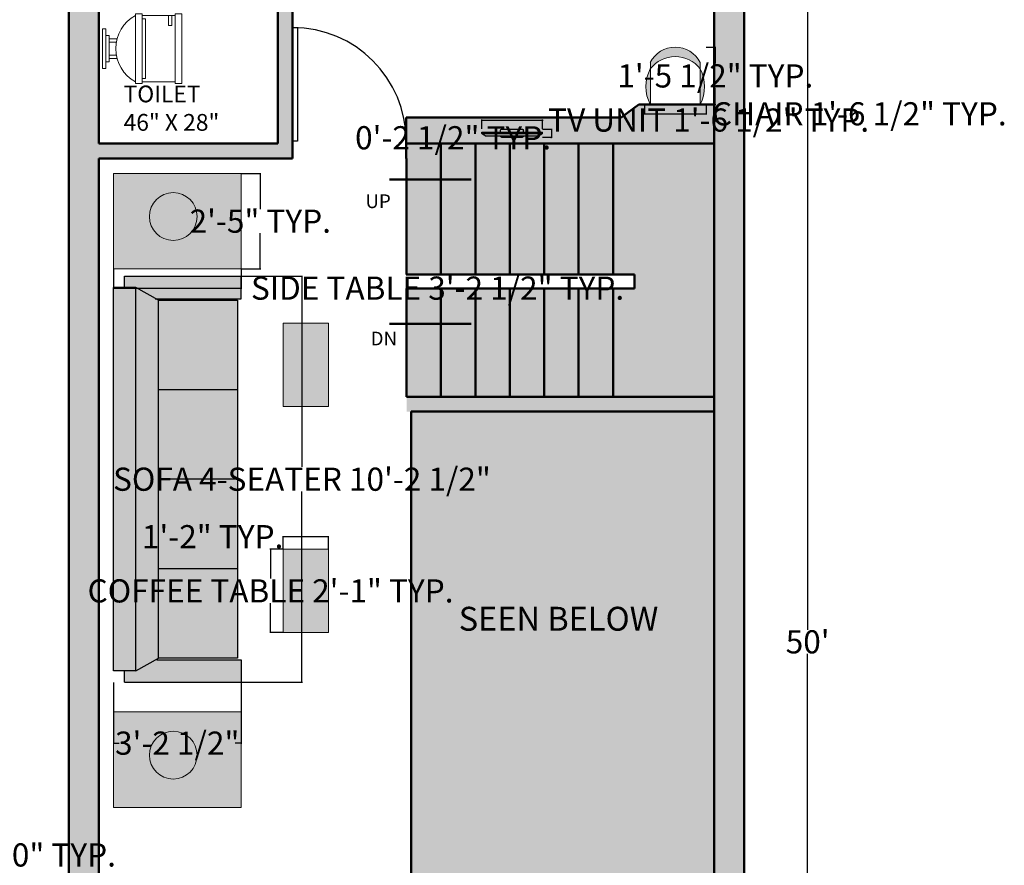
# Model space of a CAD drawing. Units: inches. Extents: x 679 to 1269, y 101 to 755.
# Tile 5 of 6: x 971 to 1269, y 370 to 626. Entities that reach past the tile are written whole.
import ezdxf

# ---------------------------------------------------------------- set-up
doc = ezdxf.new("R2010")
doc.units = ezdxf.units.IN
doc.header["$MEASUREMENT"] = 0
for name, color, linetype, lineweight in [('A-ANNO-DIMS', 2, 'Continuous', 18), ('A-ANNO-TEXT', 7, 'Continuous', 25), ('A-AREA-IDEN', 7, 'Continuous', 25), ('A-DOOR', 4, 'Continuous', 25), ('A-FLOR-FIXT', 8, 'Continuous', 18), ('A-FLOR-PATT', 8, 'Continuous', 13), ('A-FURN', 32, 'Continuous', 18), ('A-FURN-PATT', 252, 'Continuous', 13), ('A-GLAZ', 4, 'Continuous', 25), ('A-WALL', 7, 'Continuous', 50), ('A-WALL-PATT', 8, 'Continuous', 13)]:
    doc.layers.add(name, color=color, linetype=linetype, lineweight=lineweight)
doc.layers.add('furniture', color=32, linetype='Continuous')
doc.styles.get("Standard").update_dxf_attribs({"font": 'arial.ttf'})
doc.dimstyles.get("Standard").update_dxf_attribs({"dimtxt": 7, "dimasz": 0.18, "dimexe": 0.18, "dimexo": 0.0625, "dimgap": 0.09, "dimtad": 0, "dimtih": 1, "dimtoh": 1, "dimzin": 0, "dimdsep": 46, "dimlunit": 3, "dimtxsty": 'Standard', "dimcen": 0.09, "dimadec": 0, "dimazin": 0, "dimtfac": 1, "dimtofl": 0, "dimtmove": 0, "dimatfit": 3, "dimfxl": 1, "dimtolj": 1, "dimtzin": 0, "dimarcsym": 0})

# ---------------------------------------------------------------- blocks, each defined once
blk = doc.blocks.new('FABRIC SOFA 4S')
at = {"layer": 'furniture'}
for p, q in [((3, 54), (34, 54)), ((3, 51), (3, 54)), ((34, 48), (34, 54)), ((0, -51), (0, 51)), ((6, 51), (0, 51)), ((6, -51), (6, 51)), ((12, 47.63), (6, 51)), ((11.14, 48), (34, 48)), ((33, 23.81), (12, 23.81)), ((33, 0), (12, 0)), ((33, -23.81), (12, -23.81)), ((6, -51), (12, -47.63)), ((11.54, -48), (34, -48)), ((34, -48), (34, -54)), ((6, -51), (0, -51)), ((3, -54), (3, -51)), ((3, -54), (34, -54))]:
    blk.add_line(p, q, dxfattribs=at)
blk.add_lwpolyline([(12, -47.63), (12, 47.63), (33, 47.63), (33, -47.63)], close=True, dxfattribs=at)
blk = doc.blocks.new('*U4')
for p, q in [((0, 0), (0, -6)), ((40, 0), (40, -6))]:
    blk.add_line(p, q)
blk.add_lwpolyline([(0, 0), (0, 40), (1.75, 40), (1.75, 0)], close=True)
blk.add_arc((0, 0), 40, 0, 90)
blk = doc.blocks.new('*U12')
for p, q in [((-10, 22), (-10, 12)), ((-10, 21), (-7, 21)), ((-7, 21), (-7, 20)), ((10, 12), (10, 22)), ((-7, 20), (-10, 20)), ((10.5, 12), (-10.5, 12)), ((-10.5, 10), (-10.5, 12)), ((9, 13), (-9, 13)), ((-9, 13), (-9, 12)), ((9, 12), (9, 13)), ((10.5, 12), (10.5, 10)), ((10.5, 10), (-10.5, 10)), ((-3, 4.4065), (-3, 2)), ((-2, 2), (-2, 4.1658)), ((2, 4.1658), (2, 2)), ((3, 2), (3, 4.4065)), ((4, 2), (-4, 2)), ((-4, 2), (-4, 1)), ((4, 1), (4, 2))]:
    blk.add_line(p, q)
for points in [[(10.5, 22), (10.5, 24), (-10.5, 24), (-10.5, 22)], [(6, 0), (6, 1), (-6, 1), (-6, 0)]]:
    blk.add_lwpolyline(points, close=True)
blk.add_arc((0, 15.3333), 11.3333, 208.0725, 331.9275)
blk = doc.blocks.new('PLASMA-LARGE')
at = {"layer": 'furniture'}
for p, q in [((-7.26, 0), (7.26, 0)), ((-21, -2.5), (21, -2.5)), ((-21, -2.5), (-21, -3.5)), ((-21, -3.5), (21, -3.5)), ((-18.61, -1), (18.61, -1)), ((-8, -1), (-8, -0.74)), ((-8, -3.5), (-8, -4.76)), ((-7.26, -5.5), (7.26, -5.5)), ((8, -1), (8, -0.74)), ((8, -3.5), (8, -4.76)), ((21, -2.5), (21, -3.5))]:
    blk.add_line(p, q, dxfattribs=at)
for centre, radius, start, end in [((-7.26, -0.74), 0.744, 90, 180), ((7.26, -0.74), 0.744, 0, 90), ((-13.97, -11.05), 11.07, 114.76019, 129.41749), ((-7.26, -4.76), 0.744, 180, 270), ((7.26, -4.76), 0.744, 270, 0), ((13.97, -11.05), 11.07, 50.58251, 65.23981)]:
    blk.add_arc(centre, radius, start, end, dxfattribs=at)
blk = doc.blocks.new('*D16')
at = {"layer": 'A-ANNO-DIMS', "color": 0, "lineweight": -2, "transparency": 16777216}
for p, q in [((1208.37, 737.73), (1209.33, 737.73)), ((1209.15, 737.55), (1209.15, 441.39)), ((1209.15, 137.91), (1209.15, 434.07)), ((1208.37, 137.73), (1209.33, 137.73))]:
    blk.add_line(p, q, dxfattribs=at)
at = {"layer": 'A-ANNO-DIMS', "color": 0, "transparency": 16777216}
for points in [[(1209.12, 737.55), (1209.18, 737.55), (1209.15, 737.73)], [(1209.12, 137.91), (1209.18, 137.91), (1209.15, 137.73)]]:
    blk.add_solid(points, dxfattribs=at)
at = {"layer": 'Defpoints', "color": 0, "transparency": 16777216}
for p in [(1208.3, 737.73), (1208.3, 137.73), (1209.15, 137.73)]:
    blk.add_point(p, dxfattribs=at)
at = {"layer": 'A-ANNO-DIMS', "color": 0, "transparency": 16777216, "insert": (1209.15, 437.73), "char_height": 7, "attachment_point": 5}
blk.add_mtext("\\A1;50'", dxfattribs=at)
blk = doc.blocks.new('CHAIR')
h = blk.add_hatch(color=256)
h.dxf.hatch_style = 1
h.paths.add_polyline_path([(1.35, 12.72), (1.35, 10.82, -0.490483), (16.4, 10.82), (16.4, 12.72, 0.611129)])
h.paths.add_polyline_path([(1.35, 10.82, 0.248963), (1.35, 0)])
h.paths.add_polyline_path([(16.4, 10.82), (16.4, 0, 0.248963)])
for p, q in [((1.35, 12.72), (1.35, 0)), ((16.4, 12.72), (16.4, 0))]:
    blk.add_line(p, q)
for centre, radius, start, end in [((8.87, 8.86), 8.46, 27.1394, 152.8606), ((8.87, 4.99), 9.52, 37.7457, 142.2543), ((11.54, 5.41), 11.54, 152.0394, 207.9606), ((6.21, 5.41), 11.54, 332.0394, 27.9606)]:
    blk.add_arc(centre, radius, start, end)
blk = doc.blocks.new('SIDE-TABLE')
for p, q in [((0, 28.87), (38.6, 28.87)), ((0, 0), (0, 28.87)), ((38.6, 28.87), (38.6, 0)), ((38.6, 0), (0, 0))]:
    blk.add_line(p, q)
blk.add_circle((18.09, 15.83), 7.22)
blk = doc.blocks.new('COFFEE-TABLE')
for p, q in [((0, 25.18), (13.77, 25.18)), ((0, 0), (0, 25.18)), ((13.77, 25.18), (13.77, 0)), ((13.77, 0), (0, 0))]:
    blk.add_line(p, q)
blk = doc.blocks.new('*D27')
at = {"layer": 'A-ANNO-DIMS', "color": 0, "lineweight": -2, "transparency": 16777216}
for p, q in [((854.14, 376.61), (854.14, 373.18)), ((876.23, 376.61), (876.23, 373.18)), ((854.32, 373.36), (876.05, 373.36)), ((876.23, 373.36), (876.41, 373.36))]:
    blk.add_line(p, q, dxfattribs=at)
at = {"layer": 'A-ANNO-DIMS', "color": 0, "transparency": 16777216}
for points in [[(854.32, 373.39), (854.32, 373.33), (854.14, 373.36)], [(876.05, 373.39), (876.05, 373.33), (876.23, 373.36)]]:
    blk.add_solid(points, dxfattribs=at)
at = {"layer": 'Defpoints', "color": 0, "transparency": 16777216}
for p in [(854.14, 376.67), (876.23, 376.67), (876.23, 373.36)]:
    blk.add_point(p, dxfattribs=at)
at = {"layer": 'A-ANNO-DIMS', "color": 0, "transparency": 16777216, "insert": (940.47, 373.36), "char_height": 7, "attachment_point": 5}
blk.add_mtext('\\A1;SOFA 1-SEATER 1\'-10" TYP.', dxfattribs=at)
blk = doc.blocks.new('*D35')
at = {"layer": 'A-ANNO-DIMS', "color": 0, "lineweight": -2, "transparency": 16777216}
for p, q in [((1110.65, 592.61), (1110.65, 595.48)), ((1110.83, 595.3), (1128.83, 595.3)), ((1129.01, 592.61), (1129.01, 595.48)), ((1129.01, 595.3), (1129.19, 595.3))]:
    blk.add_line(p, q, dxfattribs=at)
at = {"layer": 'A-ANNO-DIMS', "color": 0, "transparency": 16777216}
for points in [[(1110.83, 595.33), (1110.83, 595.27), (1110.65, 595.3)], [(1128.83, 595.33), (1128.83, 595.27), (1129.01, 595.3)]]:
    blk.add_solid(points, dxfattribs=at)
at = {"layer": 'Defpoints', "color": 0, "transparency": 16777216}
for p in [(1129.01, 595.3), (1110.65, 592.55), (1129.01, 592.55)]:
    blk.add_point(p, dxfattribs=at)
at = {"layer": 'A-ANNO-DIMS', "color": 0, "transparency": 16777216, "insert": (1179.23, 595.3), "char_height": 7, "attachment_point": 5}
blk.add_mtext('\\A1;TV UNIT 1\'-6 1/2" TYP.', dxfattribs=at)
blk = doc.blocks.new('*D36')
at = {"layer": 'A-ANNO-DIMS', "color": 0, "lineweight": -2, "transparency": 16777216}
for p, q in [((1129.07, 592.55), (1131.94, 592.55)), ((1131.76, 592.37), (1131.76, 590.32)), ((1129.07, 590.14), (1131.94, 590.14)), ((1131.76, 589.96), (1131.58, 589.96)), ((1131.76, 590.14), (1131.76, 589.96))]:
    blk.add_line(p, q, dxfattribs=at)
at = {"layer": 'A-ANNO-DIMS', "color": 0, "transparency": 16777216}
for points in [[(1131.73, 592.37), (1131.79, 592.37), (1131.76, 592.55)], [(1131.73, 590.32), (1131.79, 590.32), (1131.76, 590.14)]]:
    blk.add_solid(points, dxfattribs=at)
at = {"layer": 'Defpoints', "color": 0, "transparency": 16777216}
for p in [(1129.01, 592.55), (1129.01, 590.14), (1131.76, 590.14)]:
    blk.add_point(p, dxfattribs=at)
at = {"layer": 'A-ANNO-DIMS', "color": 0, "transparency": 16777216, "insert": (1102, 589.96), "char_height": 7, "attachment_point": 5}
blk.add_mtext('\\A1;0\'-2 1/2" TYP.', dxfattribs=at)
blk = doc.blocks.new('*D39')
at = {"layer": 'A-ANNO-DIMS', "color": 0, "lineweight": -2, "transparency": 16777216}
for p, q in [((1038.01, 548.14), (1056.52, 548.14)), ((1056.34, 547.96), (1056.34, 490.55)), ((1056.34, 425.71), (1056.34, 483.12)), ((1038.01, 425.53), (1056.52, 425.53))]:
    blk.add_line(p, q, dxfattribs=at)
at = {"layer": 'A-ANNO-DIMS', "color": 0, "transparency": 16777216}
for points in [[(1056.31, 547.96), (1056.37, 547.96), (1056.34, 548.14)], [(1056.31, 425.71), (1056.37, 425.71), (1056.34, 425.53)]]:
    blk.add_solid(points, dxfattribs=at)
at = {"layer": 'Defpoints', "color": 0, "transparency": 16777216}
for p in [(1037.95, 548.14), (1056.34, 548.14), (1037.95, 425.53)]:
    blk.add_point(p, dxfattribs=at)
at = {"layer": 'A-ANNO-DIMS', "color": 0, "transparency": 16777216, "insert": (1056.34, 486.84), "char_height": 7, "attachment_point": 5}
blk.add_mtext('\\A1;SOFA 4-SEATER 10\'-2 1/2"', dxfattribs=at)
blk = doc.blocks.new('*D40')
at = {"layer": 'A-ANNO-DIMS', "color": 0, "lineweight": -2, "transparency": 16777216}
for p, q in [((999.35, 425.46), (999.35, 406.95)), ((1037.95, 425.46), (1037.95, 406.95)), ((999.53, 407.13), (1001.1, 407.13)), ((1037.77, 407.13), (1036.19, 407.13))]:
    blk.add_line(p, q, dxfattribs=at)
at = {"layer": 'A-ANNO-DIMS', "color": 0, "transparency": 16777216}
for points in [[(999.53, 407.16), (999.53, 407.1), (999.35, 407.13)], [(1037.77, 407.16), (1037.77, 407.1), (1037.95, 407.13)]]:
    blk.add_solid(points, dxfattribs=at)
at = {"layer": 'Defpoints', "color": 0, "transparency": 16777216}
for p in [(999.35, 425.53), (1037.95, 425.53), (1037.95, 407.13)]:
    blk.add_point(p, dxfattribs=at)
at = {"layer": 'A-ANNO-DIMS', "color": 0, "transparency": 16777216, "insert": (1018.65, 407.13), "char_height": 7, "attachment_point": 5}
blk.add_mtext('\\A1;3\'-2 1/2"', dxfattribs=at)
blk = doc.blocks.new('*D43')
at = {"layer": 'A-ANNO-DIMS', "color": 0, "lineweight": -2, "transparency": 16777216}
for p, q in [((1159.81, 599.92), (1159.81, 597.01)), ((1178.46, 599.92), (1178.46, 597.01)), ((1159.99, 597.19), (1178.28, 597.19)), ((1178.46, 597.19), (1178.64, 597.19))]:
    blk.add_line(p, q, dxfattribs=at)
at = {"layer": 'A-ANNO-DIMS', "color": 0, "transparency": 16777216}
for points in [[(1159.99, 597.22), (1159.99, 597.16), (1159.81, 597.19)], [(1178.28, 597.22), (1178.28, 597.16), (1178.46, 597.19)]]:
    blk.add_solid(points, dxfattribs=at)
at = {"layer": 'Defpoints', "color": 0, "transparency": 16777216}
for p in [(1159.81, 599.98), (1178.46, 599.98), (1178.46, 597.19)]:
    blk.add_point(p, dxfattribs=at)
at = {"layer": 'A-ANNO-DIMS', "color": 0, "transparency": 16777216, "insert": (1224.75, 597.19), "char_height": 7, "attachment_point": 5}
blk.add_mtext('\\A1;CHAIR 1\'-6 1/2" TYP.', dxfattribs=at)
blk = doc.blocks.new('*D44')
at = {"layer": 'A-ANNO-DIMS', "color": 0, "lineweight": -2, "transparency": 16777216}
for p, q in [((1178.52, 617.3), (1181.43, 617.3)), ((1181.25, 617.12), (1181.25, 612.35)), ((1181.25, 600.16), (1181.25, 604.93)), ((1178.52, 599.98), (1181.43, 599.98))]:
    blk.add_line(p, q, dxfattribs=at)
at = {"layer": 'A-ANNO-DIMS', "color": 0, "transparency": 16777216}
for points in [[(1181.22, 617.12), (1181.28, 617.12), (1181.25, 617.3)], [(1181.22, 600.16), (1181.28, 600.16), (1181.25, 599.98)]]:
    blk.add_solid(points, dxfattribs=at)
at = {"layer": 'Defpoints', "color": 0, "transparency": 16777216}
for p in [(1178.46, 617.3), (1181.25, 617.3), (1178.46, 599.98)]:
    blk.add_point(p, dxfattribs=at)
at = {"layer": 'A-ANNO-DIMS', "color": 0, "transparency": 16777216, "insert": (1181.25, 608.64), "char_height": 7, "attachment_point": 5}
blk.add_mtext('\\A1;1\'-5 1/2" TYP.', dxfattribs=at)
blk = doc.blocks.new('*D45')
at = {"layer": 'A-ANNO-DIMS', "color": 0, "lineweight": -2, "transparency": 16777216}
for p, q in [((999.35, 550.27), (999.35, 544.36)), ((1037.95, 550.28), (1037.95, 544.37)), ((999.53, 544.54), (1037.77, 544.55)), ((1037.95, 544.55), (1038.13, 544.55))]:
    blk.add_line(p, q, dxfattribs=at)
at = {"layer": 'A-ANNO-DIMS', "color": 0, "transparency": 16777216}
for points in [[(999.53, 544.57), (999.53, 544.51), (999.35, 544.54)], [(1037.77, 544.58), (1037.77, 544.52), (1037.95, 544.55)]]:
    blk.add_solid(points, dxfattribs=at)
at = {"layer": 'Defpoints', "color": 0, "transparency": 16777216}
for p in [(999.35, 550.33), (1037.95, 550.34), (1037.95, 544.55)]:
    blk.add_point(p, dxfattribs=at)
at = {"layer": 'A-ANNO-DIMS', "color": 0, "transparency": 16777216, "insert": (1097.32, 544.55), "char_height": 7, "attachment_point": 5}
blk.add_mtext('\\A1;SIDE TABLE 3\'-2 1/2" TYP.', dxfattribs=at)
blk = doc.blocks.new('*D46')
at = {"layer": 'A-ANNO-DIMS', "color": 0, "lineweight": -2, "transparency": 16777216}
for p, q in [((1038.01, 579.21), (1043.91, 579.21)), ((1043.73, 579.03), (1043.74, 568.44)), ((1043.74, 550.53), (1043.74, 561.11)), ((1038.02, 550.34), (1043.92, 550.35))]:
    blk.add_line(p, q, dxfattribs=at)
at = {"layer": 'A-ANNO-DIMS', "color": 0, "transparency": 16777216}
for points in [[(1043.76, 579.03), (1043.7, 579.03), (1043.73, 579.21)], [(1043.77, 550.53), (1043.71, 550.53), (1043.74, 550.35)]]:
    blk.add_solid(points, dxfattribs=at)
at = {"layer": 'Defpoints', "color": 0, "transparency": 16777216}
for p in [(1037.94, 579.21), (1043.73, 579.21), (1037.95, 550.34)]:
    blk.add_point(p, dxfattribs=at)
at = {"layer": 'A-ANNO-DIMS', "color": 0, "transparency": 16777216, "insert": (1043.74, 564.78), "char_height": 7, "attachment_point": 5}
blk.add_mtext('\\A1;2\'-5" TYP.', dxfattribs=at)
blk = doc.blocks.new('*D47')
at = {"layer": 'A-ANNO-DIMS', "color": 0, "lineweight": -2, "transparency": 16777216}
for p, q in [((1050.55, 465.7), (1046.66, 465.7)), ((1046.84, 465.52), (1046.84, 456.82)), ((1046.84, 440.7), (1046.84, 449.4)), ((1050.55, 440.52), (1046.66, 440.52))]:
    blk.add_line(p, q, dxfattribs=at)
at = {"layer": 'A-ANNO-DIMS', "color": 0, "transparency": 16777216}
for points in [[(1046.81, 465.52), (1046.87, 465.52), (1046.84, 465.7)], [(1046.81, 440.7), (1046.87, 440.7), (1046.84, 440.52)]]:
    blk.add_solid(points, dxfattribs=at)
at = {"layer": 'Defpoints', "color": 0, "transparency": 16777216}
for p in [(1050.61, 465.7), (1046.84, 440.52), (1050.61, 440.52)]:
    blk.add_point(p, dxfattribs=at)
at = {"layer": 'A-ANNO-DIMS', "color": 0, "transparency": 16777216, "insert": (1046.84, 453.11), "char_height": 7, "attachment_point": 5}
blk.add_mtext('\\A1;COFFEE TABLE 2\'-1" TYP.', dxfattribs=at)
blk = doc.blocks.new('*D48')
at = {"layer": 'A-ANNO-DIMS', "color": 0, "lineweight": -2, "transparency": 16777216}
for p, q in [((1050.61, 469.48), (1050.43, 469.48)), ((1050.61, 465.76), (1050.61, 469.66)), ((1064.2, 469.48), (1050.79, 469.48)), ((1064.38, 465.76), (1064.38, 469.66))]:
    blk.add_line(p, q, dxfattribs=at)
at = {"layer": 'A-ANNO-DIMS', "color": 0, "transparency": 16777216}
for points in [[(1050.79, 469.51), (1050.79, 469.45), (1050.61, 469.48)], [(1064.2, 469.51), (1064.2, 469.45), (1064.38, 469.48)]]:
    blk.add_solid(points, dxfattribs=at)
at = {"layer": 'Defpoints', "color": 0, "transparency": 16777216}
for p in [(1050.61, 469.48), (1050.61, 465.7), (1064.38, 465.7)]:
    blk.add_point(p, dxfattribs=at)
at = {"layer": 'A-ANNO-DIMS', "color": 0, "transparency": 16777216, "insert": (1029.34, 469.48), "char_height": 7, "attachment_point": 5}
blk.add_mtext('\\A1;1\'-2" TYP.', dxfattribs=at)

msp = doc.modelspace()

# ---------------------------------------------------------------- hatches: boundary and pattern name
at = {"layer": 'A-FLOR-PATT'}
h = msp.add_hatch(dxfattribs=at)
h.set_pattern_fill('ANSI31', color=256)
h.paths.add_polyline_path([(1119.805, 251.542), (1104.539, 251.542), (1104.539, 181.227), (1119.805, 181.227)])
h.paths.add_polyline_path([(1111.468, 194.139), (1110.457, 194.139), (1110.457, 207.286), (1109.187, 207.286, -0.4142136), (1108.434, 208.038), (1108.434, 222.713, -0.4142136), (1109.187, 223.466), (1110.457, 223.466), (1110.457, 236.613), (1111.468, 236.613, -0.0640419), (1112.985, 234.194), (1112.985, 223.466), (1113.243, 223.466, -0.4142136), (1113.996, 222.713), (1113.996, 208.038, -0.4142136), (1113.243, 207.286), (1112.985, 207.286), (1112.985, 196.558, -0.0640419)], flags=16)
h.paths.add_polyline_path([(794.414, 488.811), (775.786, 488.811), (775.786, 449.729), (775.786, 418.496), (794.414, 418.496)])
h.paths.add_polyline_path([(785.134, 431.408), (784.123, 431.408, -0.0640419), (782.606, 433.827), (782.606, 444.555), (782.347, 444.555, -0.4142136), (781.595, 445.308), (781.595, 459.983, -0.4142136), (782.347, 460.736), (782.606, 460.736), (782.606, 471.463, -0.0640419), (784.123, 473.882), (785.134, 473.882), (785.134, 460.736), (786.404, 460.736, -0.4142136), (787.157, 459.983), (787.157, 445.308, -0.4142136), (786.404, 444.555), (785.134, 444.555)], flags=16)
at = {"layer": 'A-FURN-PATT'}
h = msp.add_hatch(color=256, dxfattribs=at)
h.dxf.hatch_style = 1
h.paths.add_polyline_path([(1180.931, 599.984), (1158.171, 599.984), (1152.762, 596.11), (1087.862, 596.11), (1087.862, 588.883), (1087.862, 588.229), (1180.931, 588.229)])
h = msp.add_hatch(color=256, dxfattribs=at)
h.dxf.hatch_style = 1
h.paths.add_polyline_path([(1130.752, 594.975), (1108.734, 594.975), (1108.734, 588.229), (1130.752, 588.229)])
h.paths.add_polyline_path([(1116.329, 591.674), (1116.329, 592.223, -0.4142136), (1116.654, 592.548), (1122.999, 592.548, -0.4142136), (1123.324, 592.223), (1123.324, 591.674), (1129.007, 591.674), (1129.007, 591.237, -0.0640419), (1127.961, 590.581), (1123.324, 590.581), (1123.324, 590.469, -0.4142136), (1122.999, 590.144), (1116.654, 590.144, -0.4142136), (1116.329, 590.469), (1116.329, 590.581), (1111.692, 590.581, -0.0640419), (1110.646, 591.237), (1110.646, 591.674)], flags=16)
h = msp.add_hatch(color=256, dxfattribs=at)
h.dxf.hatch_style = 1
h.paths.add_polyline_path([(1037.949, 548.144), (1002.753, 548.144), (1002.753, 544.738), (1006.159, 544.738), (1012.214, 541.332), (1037.949, 541.332)])
h.paths.add_polyline_path([(1037.949, 432.339), (1012.214, 432.339), (1006.159, 428.933), (1002.753, 428.933), (1002.753, 425.527), (1037.949, 425.527)])
h.paths.add_polyline_path([(1012.971, 540.906), (1006.159, 544.738), (1006.159, 428.933), (1012.971, 432.764)])
h.paths.add_polyline_path([(1006.159, 544.738), (999.347, 544.738), (999.347, 428.933), (1006.159, 428.933)])
h.paths.add_polyline_path([(1036.813, 540.906), (1012.971, 540.906), (1012.971, 513.87), (1036.813, 513.87)])
h.paths.add_polyline_path([(1036.813, 513.87), (1012.971, 513.87), (1012.971, 486.835), (1036.813, 486.835)])
h.paths.add_polyline_path([(1036.813, 486.835), (1012.971, 486.835), (1012.971, 459.8), (1036.813, 459.8)])
h.paths.add_polyline_path([(1036.813, 459.8), (1012.971, 459.8), (1012.971, 432.764), (1036.813, 432.764)])
at = {"layer": 'A-GLAZ'}
h = msp.add_hatch(color=256, dxfattribs=at)
h.dxf.hatch_style = 1
h.paths.add_polyline_path([(994.931, 583.729), (1053.502, 583.729), (1053.502, 588.883), (1053.502, 623.243), (1053.502, 645.329), (1049.002, 645.329), (1049.002, 588.229), (994.931, 588.229), (994.931, 674.229), (1053.502, 674.229), (1053.502, 678.729), (994.931, 678.729), (994.931, 728.729), (1180.931, 728.729), (1180.931, 356.354), (1033.405, 356.354), (1033.405, 351.854), (1119.805, 351.854), (1119.805, 281.2), (1124.305, 281.2), (1124.305, 351.854), (1180.931, 351.854), (1180.931, 251.542), (1161.199, 251.542), (1161.199, 247.042), (1189.931, 247.042), (1189.931, 737.729), (985.931, 737.729), (985.931, 137.729), (1015.759, 137.729), (1015.759, 146.729), (994.931, 146.729)])
h.paths.add_polyline_path([(1185.698, 247.042), (1180.931, 247.042), (1180.931, 146.729), (1124.305, 146.729), (1124.305, 142.229), (1185.698, 142.229)], flags=0)
h.paths.add_polyline_path([(1189.931, 247.042), (1185.698, 247.042), (1185.698, 142.229), (1124.305, 142.229), (1124.305, 137.729), (1189.931, 137.729)], flags=17)
at = {"layer": 'A-WALL-PATT'}
h = msp.add_hatch(color=256, dxfattribs=at)
h.dxf.hatch_style = 1
h.paths.add_polyline_path([(1189.931, 737.729), (985.931, 737.729), (985.931, 137.729), (1015.759, 137.729), (1015.759, 146.729), (994.931, 146.729), (994.931, 583.729), (1053.502, 583.729), (1053.502, 645.329), (1049.002, 645.329), (1049.002, 588.229), (994.931, 588.229), (994.931, 674.229), (1012.305, 674.229), (1012.305, 678.729), (994.931, 678.729), (994.931, 728.729), (1053.502, 728.729), (1053.502, 678.729), (1053.502, 674.229), (1049.002, 674.229), (1049.002, 645.329), (1053.502, 645.329), (1053.502, 583.729), (994.931, 583.729), (994.931, 146.729), (1180.931, 146.729), (1180.931, 247.042), (1124.305, 247.042), (1124.305, 176.159), (1119.805, 176.159), (1119.805, 181.227), (1104.539, 181.227), (1104.539, 251.542), (1119.805, 251.542), (1124.238, 251.542), (1124.238, 281.2), (1119.805, 281.2), (1119.805, 331.601), (1036.785, 331.601), (1036.785, 351.854), (1033.393, 351.854), (1033.393, 356.354), (1033.405, 356.354), (1089.362, 356.354), (1089.362, 507.268), (1180.931, 507.268), (1180.931, 356.354), (1089.362, 356.354), (1033.405, 356.354), (1033.405, 351.854), (1119.805, 351.854), (1119.805, 281.2), (1124.305, 281.2), (1124.305, 351.854), (1180.931, 351.854), (1180.931, 251.542), (1161.199, 251.542), (1161.199, 247.042), (1189.931, 247.042)], flags=17)
h.paths.add_polyline_path([(1087.931, 548.661), (1087.931, 583.729), (1087.862, 588.229), (1087.862, 583.729), (1087.931, 583.729), (1150.34, 583.729), (1150.34, 548.661)], flags=0)
h.paths.add_polyline_path([(1161.61, 599.984, -0.2489628), (1161.61, 610.804), (1161.61, 612.705, -0.611129), (1176.66, 612.705), (1176.66, 610.804, -0.2489628), (1176.66, 599.984)], flags=0)
h.paths.add_polyline_path([(1064.382, 534.011), (1064.382, 508.83), (1050.613, 508.83), (1050.613, 534.011)], flags=0)
h.paths.add_polyline_path([(1153.405, 653.658), (1150.32, 653.658), (1150.32, 654.172), (1137.85, 654.172), (1137.85, 653.658), (1134.765, 653.658), (1134.765, 669.599), (1136.307, 669.599), (1136.307, 671.141), (1131.356, 671.141), (1131.356, 669.599), (1132.898, 669.599), (1132.898, 653.658), (1129.813, 653.658), (1129.813, 654.172), (1117.343, 654.172), (1117.343, 653.658), (1114.258, 653.658), (1114.258, 669.599), (1115.801, 669.599), (1115.801, 671.141), (1112.147, 671.141), (1112.147, 669.599), (1113.69, 669.599), (1113.69, 653.658), (1110.605, 653.658), (1110.605, 654.172), (1098.135, 654.172), (1098.135, 653.658), (1095.05, 653.658), (1095.05, 669.599), (1095.05, 671.141), (1096.592, 671.141), (1112.147, 671.141), (1115.801, 671.141), (1131.356, 671.141), (1136.307, 671.141), (1151.862, 671.141), (1153.405, 671.141), (1153.405, 669.599)], flags=0)
h.paths.add_polyline_path([(1037.949, 548.144), (1037.949, 541.332), (1012.214, 541.332), (1012.971, 540.906), (1036.813, 540.906), (1036.813, 432.764), (1012.971, 432.764), (1006.159, 428.933), (999.347, 428.933), (999.347, 544.738), (1002.753, 544.738), (1002.753, 548.144)], flags=0)
h.paths.add_polyline_path([(1037.949, 550.347), (999.347, 550.347), (999.347, 579.213), (1037.949, 579.213)], flags=0)
h.paths.add_polyline_path([(1064.382, 465.7), (1064.382, 440.519), (1050.613, 440.519), (1050.613, 465.7)], flags=0)
h.paths.add_polyline_path([(1146.082, 678.097), (1096.893, 678.097), (1096.893, 698.607), (1104.314, 698.607), (1104.314, 717.374), (1096.049, 717.453), (1096.049, 726.931), (1104.314, 726.852), (1141.204, 726.852), (1149.469, 726.772), (1149.469, 717.294), (1141.204, 717.374), (1141.204, 698.607), (1146.082, 698.607)], flags=0)
h.paths.add_polyline_path([(1189.931, 737.729), (985.931, 737.729), (985.931, 137.729), (1015.759, 137.729), (1015.759, 146.729), (994.931, 146.729), (994.931, 583.729), (1053.502, 583.729), (1053.502, 645.329), (1049.002, 645.329), (1049.002, 588.229), (994.931, 588.229), (994.931, 674.229), (1012.305, 674.229), (1012.305, 678.729), (994.931, 678.729), (994.931, 728.729), (1053.502, 728.729), (1053.502, 674.229), (1049.002, 674.229), (1049.002, 645.329), (1053.502, 645.329), (1053.502, 583.729), (994.931, 583.729), (994.931, 146.729), (1180.931, 146.729), (1180.931, 247.042), (1124.305, 247.042), (1124.305, 176.159), (1119.805, 176.159), (1119.805, 181.227), (1104.539, 181.227), (1104.539, 251.542), (1119.805, 251.542), (1124.238, 251.542), (1124.238, 281.2), (1119.805, 281.2), (1119.805, 331.601), (1036.785, 331.601), (1036.785, 351.854), (1033.393, 351.854), (1033.393, 356.354), (1089.362, 356.354), (1089.362, 507.268), (1180.931, 507.268), (1180.931, 356.354), (1033.405, 356.354), (1033.405, 351.854), (1119.805, 351.854), (1119.805, 281.2), (1124.305, 281.2), (1124.305, 351.854), (1180.931, 351.854), (1180.931, 251.542), (1161.199, 251.542), (1161.199, 247.042), (1189.931, 247.042)], flags=17)
h.paths.add_polyline_path([(1087.931, 583.729), (1087.862, 583.729), (1087.862, 588.229), (1087.862, 588.883), (1087.862, 596.11), (1152.762, 596.11), (1158.171, 599.984), (1161.61, 599.984, -0.2489628), (1161.61, 610.804), (1161.61, 612.705, -0.611129), (1176.66, 612.705), (1176.66, 610.804, -0.2489628), (1176.66, 599.984), (1161.61, 599.984), (1158.171, 599.984), (1152.762, 596.11), (1087.862, 596.11), (1087.862, 588.883), (1087.862, 588.229), (1087.931, 583.729), (1150.34, 583.729), (1150.34, 548.661), (1087.931, 548.661)], flags=0)
h.paths.add_polyline_path([(1087.931, 583.729), (1087.862, 588.229), (1087.862, 583.729), (1150.34, 583.729), (1150.34, 548.661), (1087.931, 548.661)], flags=0)
h.paths.add_polyline_path([(1161.61, 610.804), (1161.61, 612.705, -0.611129), (1176.66, 612.705), (1176.66, 610.804, -0.2489628), (1176.66, 599.984), (1176.66, 610.804, 0.4904831), (1161.61, 610.804), (1161.61, 599.984, -0.2489628)], flags=0)
h = msp.add_hatch(color=256, dxfattribs=at)
h.dxf.hatch_style = 1
h.paths.add_polyline_path([(1180.931, 507.268), (1089.362, 507.268), (1089.362, 356.354), (1180.931, 356.354)])
h.paths.add_polyline_path([(1037.949, 416.536), (999.347, 416.536), (999.347, 387.67), (1037.949, 387.67)])
h.paths.add_polyline_path([(1037.949, 579.213), (999.347, 579.213), (999.347, 550.347), (1037.949, 550.347)])
h.paths.add_polyline_path([(1064.382, 465.7), (1050.613, 465.7), (1050.613, 440.519), (1064.382, 440.519)])
h.paths.add_polyline_path([(1064.382, 534.011), (1050.613, 534.011), (1050.613, 508.83), (1064.382, 508.83)])
h.paths.add_polyline_path([(1017.114, 194.268), (1003.506, 194.268), (1003.391, 182.402), (1010.195, 182.402), (1010.195, 183.635, -0.4142136), (1005.815, 188.015, -1), (1014.576, 188.015, -0.4142136), (1010.195, 183.635), (1010.195, 182.402), (1017, 182.402)])
h.paths.add_polyline_path([(1014.691, 252.849, -0.4142136), (1010.31, 248.468), (1010.31, 247.235), (1017.114, 247.235), (1017.229, 259.102), (1003.62, 259.102), (1003.506, 247.235), (1010.31, 247.235), (1010.31, 248.468, -0.4142136), (1005.929, 252.849, -1)])
h.paths.add_polyline_path([(1104.314, 726.852), (1096.049, 726.931), (1096.049, 722.192), (1096.908, 722.192, -1), (1103.01, 722.192, -1), (1096.908, 722.192), (1096.049, 722.192), (1096.049, 717.453), (1104.314, 717.374)])
h.paths.add_polyline_path([(1149.469, 726.772), (1141.204, 726.852), (1141.204, 722.113), (1142.063, 722.113, -1), (1148.165, 722.113, -1), (1142.063, 722.113), (1141.204, 722.113), (1141.204, 717.374), (1149.469, 717.294)])
h.paths.add_polyline_path([(826.598, 726.852), (818.333, 726.931), (818.333, 722.192), (819.192, 722.192, -1), (825.294, 722.192, -1), (819.192, 722.192), (818.333, 722.192), (818.333, 717.453), (826.598, 717.374)])
h.paths.add_polyline_path([(871.752, 726.772), (863.487, 726.852), (863.487, 722.113), (864.346, 722.113, -1), (870.448, 722.113, -1), (864.346, 722.113), (863.487, 722.113), (863.487, 717.374), (871.752, 717.294)])
h = msp.add_hatch(color=256, dxfattribs=at)
h.dxf.hatch_style = 1
h.paths.add_polyline_path([(1180.931, 588.229), (1150.34, 588.229), (1150.34, 583.729), (1150.34, 548.661), (1156.809, 548.661), (1156.809, 544.406), (1150.34, 544.406), (1150.34, 511.729), (1180.931, 511.729)])
h.paths.add_polyline_path([(1150.34, 583.729), (1150.34, 588.19), (1139.939, 588.19), (1139.939, 548.661), (1150.34, 548.661)])
h.paths.add_polyline_path([(1139.939, 588.19), (1129.537, 588.19), (1129.537, 548.661), (1139.939, 548.661)])
h.paths.add_polyline_path([(1129.537, 588.19), (1119.135, 588.19), (1119.135, 548.661), (1129.537, 548.661)])
h.paths.add_polyline_path([(1119.135, 588.19), (1108.734, 588.19), (1108.734, 548.661), (1119.135, 548.661)])
h.paths.add_polyline_path([(1108.734, 588.19), (1098.332, 588.19), (1098.332, 583.729), (1098.332, 548.661), (1108.734, 548.661)])
h.paths.add_polyline_path([(1098.332, 583.729), (1098.332, 588.19), (1087.862, 588.19), (1087.862, 583.729), (1087.931, 583.729), (1087.931, 548.661), (1098.332, 548.661)])
h.paths.add_polyline_path([(1150.34, 544.406), (1139.939, 544.406), (1139.939, 511.729), (1150.34, 511.729)])
h.paths.add_polyline_path([(1139.939, 544.406), (1129.537, 544.406), (1129.537, 511.729), (1139.939, 511.729)])
h.paths.add_polyline_path([(1129.537, 544.406), (1119.135, 544.406), (1119.135, 511.729), (1129.537, 511.729)])
h.paths.add_polyline_path([(1119.135, 544.406), (1108.734, 544.406), (1108.734, 511.729), (1119.135, 511.729)])
h.paths.add_polyline_path([(1108.734, 544.406), (1098.332, 544.406), (1098.332, 511.729), (1108.734, 511.729)])
h.paths.add_polyline_path([(1098.332, 544.406), (1087.931, 544.406), (1087.931, 511.729), (1098.332, 511.729)])
h = msp.add_hatch(color=256, dxfattribs=at)
h.dxf.hatch_style = 1
h.paths.add_polyline_path([(1024.651, 403.502, 1), (1010.216, 403.502, 1)])
h.paths.add_polyline_path([(1010.216, 566.134, 1), (1024.651, 566.134, 1)])
h = msp.add_hatch(color=256, dxfattribs=at)
h.dxf.hatch_style = 1
h.paths.add_polyline_path([(1180.931, 511.729), (1087.931, 511.729), (1087.931, 507.229), (1180.931, 507.229)])

# ---------------------------------------------------------------- linework, layer by layer
at = {"layer": 'A-WALL'}
for p, q in [((985.931, 137.729), (985.931, 737.729)), ((1189.931, 737.729), (1189.931, 137.729)), ((1180.931, 728.729), (1180.931, 356.354)), ((994.931, 588.229), (994.931, 674.229)), ((1049.002, 588.229), (1049.002, 674.229)), ((1053.502, 583.729), (1053.502, 645.329)), ((1152.762, 596.11), (1158.171, 599.984)), ((1158.171, 599.984), (1180.931, 599.984)), ((1087.862, 588.883), (1087.862, 596.11)), ((1087.862, 596.11), (1152.762, 596.11)), ((994.931, 588.229), (1049.002, 588.229)), ((1087.862, 588.883), (1087.862, 588.229)), ((1087.862, 588.229), (1087.862, 583.729)), ((1098.332, 588.19), (1087.862, 588.19)), ((1087.862, 588.19), (1150.34, 588.19)), ((1098.332, 588.19), (1098.332, 548.661)), ((1098.332, 583.729), (1098.332, 588.19)), ((1108.734, 588.19), (1108.734, 548.661)), ((1119.135, 588.19), (1119.135, 548.661)), ((1129.537, 588.19), (1129.537, 548.661)), ((1139.939, 588.19), (1139.939, 548.661)), ((1180.931, 588.229), (1150.34, 588.229)), ((1150.34, 588.19), (1150.34, 548.661)), ((1150.34, 588.19), (1150.34, 583.729)), ((1180.931, 511.729), (1180.931, 588.229)), ((994.931, 146.729), (994.931, 583.729)), ((994.931, 583.729), (1053.502, 583.729)), ((1087.931, 583.729), (1087.931, 548.661)), ((1082.755, 577.34), (1107.427, 577.34)), ((1087.862, 548.661), (1156.809, 548.661)), ((1156.809, 548.661), (1156.809, 544.406)), ((1156.809, 544.406), (1087.862, 544.406)), ((1087.931, 544.406), (1087.931, 511.729)), ((1098.332, 544.406), (1098.332, 511.729)), ((1108.734, 544.406), (1108.734, 511.729)), ((1119.135, 544.406), (1119.135, 511.729)), ((1129.537, 544.406), (1129.537, 511.729)), ((1139.939, 544.406), (1139.939, 511.729)), ((1150.34, 544.406), (1150.34, 511.729)), ((1082.755, 533.743), (1107.427, 533.743)), ((1087.931, 511.729), (1180.931, 511.729)), ((1089.362, 507.268), (1089.362, 356.354)), ((1089.362, 507.268), (1180.931, 507.268)), ((1180.931, 507.268), (1180.931, 356.354))]:
    msp.add_line(p, q, dxfattribs=at)

# ---------------------------------------------------------------- block references
at = {"layer": 'A-DOOR', "xscale": 0.8589852122862605, "yscale": 0.8589852122862605, "zscale": 0.8589852122862605}
msp.add_blockref('*U4', (1053.502, 588.883), dxfattribs=at)
at = {"layer": 'A-FLOR-FIXT', "rotation": 269.9999999999999}
msp.add_blockref('*U12', (996.046, 616.875), dxfattribs=at)
at = {"layer": 'A-FURN'}
for name, p in [('CHAIR', (1160.263, 599.984)), ('COFFEE-TABLE', (1050.613, 508.83)), ('SIDE-TABLE', (999.347, 387.67))]:
    msp.add_blockref(name, p, dxfattribs=at)
at = {"layer": 'A-FURN', "xscale": -0.4371808821614596, "yscale": 0.4371808821614596, "zscale": 0.4371808821614596, "rotation": 180}
msp.add_blockref('PLASMA-LARGE', (1119.827, 590.144), dxfattribs=at)
at = {"layer": 'A-FURN'}
for name, p, rotation in [('SIDE-TABLE', (999.351, 550.332), 0.0169632942639133), ('COFFEE-TABLE', (1064.382, 465.7), 180)]:
    msp.add_blockref(name, p, dxfattribs=dict(at, rotation=rotation))
at = {"layer": 'A-FURN', "xscale": 1.135342513121085, "yscale": 1.135342513121085, "zscale": 1.135342513121085}
msp.add_blockref('FABRIC SOFA 4S', (999.347, 486.835), dxfattribs=at)

# ---------------------------------------------------------------- texts
at = {"layer": 'A-ANNO-TEXT'}
for s, p in [('UP', (1075.517, 568.715)), ('DN', (1077.089, 527.253))]:
    msp.add_text(s, height=4.1487, dxfattribs=at).set_placement(p)
at = {"layer": 'A-AREA-IDEN'}
for s, height, p in [('TOILET', 5.065, (1002.423, 600.664)), ('46" X 28"', 5.065, (1002.423, 592.069)), ('SEEN BELOW', 7.213, (1103.701, 441.09))]:
    msp.add_text(s, height=height, dxfattribs=at).set_placement(p)

# ---------------------------------------------------------------- dimensions: what is measured, and where the dimension line sits
at = {"layer": 'A-ANNO-DIMS'}
dim = msp.add_linear_dim(base=(1209.153, 137.729), p1=(1208.303, 737.729), p2=(1208.303, 137.729), angle=90, dimstyle='Standard', override={"dimclrd": 0, "dimclre": 0, "dimclrt": 0}, dxfattribs=at)
dim.commit()
dim.dimension.update_dxf_attribs({"geometry": '*D16', "text_midpoint": (1209.153, 437.729)})
for base, p1, p2, angle, text, picture, middle in [((1181.252, 617.304), (1178.456, 599.984), (1178.456, 617.304), 90, '<> TYP.', '*D44', (1181.252, 608.644)), ((1131.762, 590.144), (1129.007, 592.548), (1129.007, 590.144), 270, '<> TYP.', '*D36', (1102.002, 589.964)), ((1043.735, 579.211), (1037.953, 550.344), (1037.945, 579.21), 90.01696, '<> TYP.', '*D46', (1043.739, 564.778)), ((1037.955, 544.554), (999.351, 550.332), (1037.953, 550.344), 0.01696, 'SIDE TABLE <> TYP.', '*D45', (1097.317, 544.554)), ((1056.341, 548.144), (1037.949, 425.527), (1037.949, 548.144), 90, 'SOFA 4-SEATER <>', '*D39', (1056.341, 486.835)), ((1050.613, 469.477), (1064.382, 465.7), (1050.613, 465.7), 180, '<> TYP.', '*D48', (1029.339, 469.477)), ((1046.836, 440.519), (1050.613, 465.7), (1050.613, 440.519), 270, 'COFFEE TABLE <> TYP.', '*D47', (1046.836, 453.11))]:
    dim = msp.add_linear_dim(base=base, p1=p1, p2=p2, angle=angle, text=text, dimstyle='Standard', override={"dimdec": 1, "dimrnd": 0, "dimzin": 1, "dimlunit": 4, "dimfrac": 2}, dxfattribs=at)
    dim.commit()
    dim.dimension.update_dxf_attribs({"geometry": picture, "text_midpoint": middle})
for base, p1, p2, text, picture, middle in [((1129.007, 595.302), (1110.646, 592.548), (1129.007, 592.548), 'TV UNIT <> TYP.', '*D35', (1179.228, 595.302)), ((1178.456, 597.188), (1159.814, 599.984), (1178.456, 599.984), 'CHAIR <> TYP.', '*D43', (1224.746, 597.188)), ((876.227, 373.358), (854.135, 376.671), (876.227, 376.671), 'SOFA 1-SEATER <> TYP.', '*D27', (940.473, 373.358))]:
    dim = msp.add_linear_dim(base=base, p1=p1, p2=p2, text=text, dimstyle='Standard', override={"dimdec": 1, "dimrnd": 0, "dimzin": 1, "dimlunit": 4, "dimfrac": 2}, dxfattribs=at)
    dim.commit()
    dim.dimension.update_dxf_attribs({"geometry": picture, "text_midpoint": middle})
dim = msp.add_linear_dim(base=(1037.949, 407.134), p1=(999.347, 425.527), p2=(1037.949, 425.527), dimstyle='Standard', override={"dimdec": 1, "dimrnd": 0, "dimzin": 1, "dimlunit": 4, "dimfrac": 2}, dxfattribs=at)
dim.commit()
dim.dimension.update_dxf_attribs({"geometry": '*D40', "text_midpoint": (1018.648, 407.134)})

doc.saveas('drawing.dxf')
